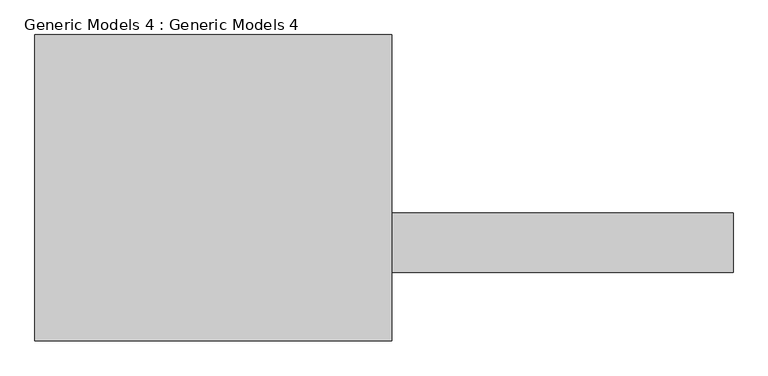
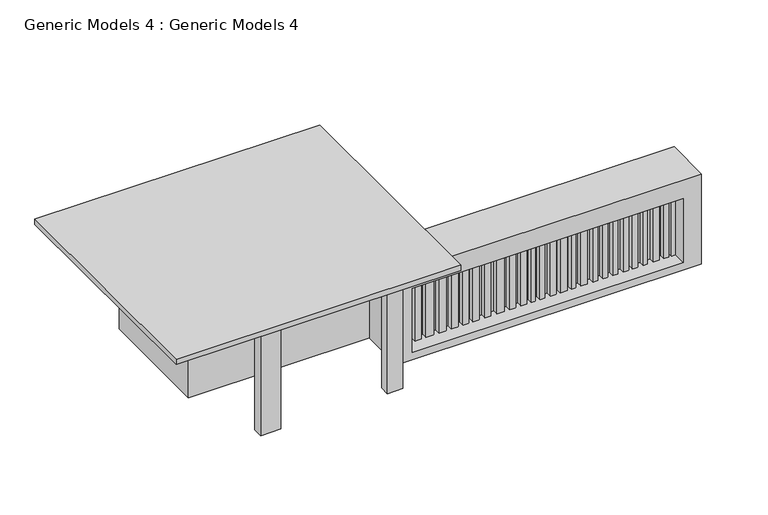
"""IFC4 building model written with IfcOpenShell, lengths in millimetres: proxy geometry, Generic Models 4 : Generic Models 4."""

from ifc_helpers import new_model, si_unit, frame, origin, place, context, project, spatial, polyline, outline, extrude, faceted_brep, source, transform, mapped, element, save


def generic_models_4_generic_models_4_f36dcc8b(model_context):
    return source(origin(), model_context, "Body", "SolidModel", [
        extrude(outline(polyline([(1788.9557244, -13852.2176249), (-4615.7230912, -13852.2176249), (-4615.7230912, -8353.4436591), (1788.9557244, -8353.4436591), (1788.9557244, -13852.2176249)])), frame((0.0, 0.0, 9144.0), z_axis=(0.0, 0.0, 1.0), x_axis=(1.0, 0.0, 0.0)), (0.0, 0.0, 1.0), 127.0),
        extrude(outline(polyline([(413.7770384, -13376.4602599), (413.7770384, -13147.8602599), (763.5531931, -13147.8602599), (763.5531931, -13376.4602599), (413.7770384, -13376.4602599)])), frame((0.0, 0.0, 6400.8), z_axis=(0.0, 0.0, 1.0), x_axis=(1.0, 0.0, 0.0)), (0.0, 0.0, 1.0), 2743.2),
        extrude(outline(polyline([(-2439.060811, -13147.8602599), (-1981.860811, -13147.8602599), (-1981.860811, -13376.4602599), (-2439.060811, -13376.4602599), (-2439.060811, -13147.8602599)])), frame((0.0, 0.0, 6400.8), z_axis=(0.0, 0.0, 1.0), x_axis=(1.0, 0.0, 0.0)), (0.0, 0.0, 1.0), 2743.2),
        extrude(outline(polyline([(-3010.560811, -11553.8436591), (-3010.560811, -8857.8706536), (1058.1030034, -8857.8706536), (1058.1030034, -11553.8436591), (-3010.560811, -11553.8436591)])), frame((0.0, 0.0, 6400.8), z_axis=(0.0, 0.0, 1.0), x_axis=(1.0, 0.0, 0.0)), (0.0, 0.0, 1.0), 2743.2),
        faceted_brep([(1058.1030034, -12620.6436591, 8549.4766171), (7916.1030034, -12620.6436591, 8549.4766171), (7916.1030034, -11553.8436591, 8549.4766171), (1058.1030034, -11553.8436591, 8549.4766171), (1058.1030034, -12620.6436591, 6400.8), (1058.1030034, -11553.8436591, 6400.8), (7916.1030034, -11553.8436591, 6400.8), (7916.1030034, -12620.6436591, 6400.8), (7505.039189, -12620.6436591, 8103.1737426), (7505.039189, -12620.6436591, 6579.1737426), (1409.039189, -12620.6436591, 6579.1737426), (1409.039189, -12620.6436591, 8103.1737426), (1409.039189, -12315.8436591, 8103.1737426), (1409.039189, -12315.8436591, 6579.1737426), (1527.4997407, -12315.8436591, 6579.1737426), (1527.4997407, -12315.8436591, 8103.1737426), (7505.039189, -12315.8436591, 6579.1737426), (7505.039189, -12315.8436591, 8103.1737426), (7412.689646, -12315.8436591, 8103.1737426), (7412.689646, -12315.8436591, 6579.1737426), (1788.9557244, -12315.8436591, 8103.1737426), (1637.639189, -12315.8436591, 8103.1737426), (1637.639189, -12315.8436591, 6579.1737426), (1788.9557244, -12315.8436591, 6579.1737426), (2067.842107, -12315.8436591, 8103.1737426), (1893.5381178, -12315.8436591, 8103.1737426), (1893.5381178, -12315.8436591, 6579.1737426), (2067.842107, -12315.8436591, 6579.1737426), (2346.7284896, -12315.8436591, 8103.1737426), (2181.1396999, -12315.8436591, 8103.1737426), (2181.1396999, -12315.8436591, 6579.1737426), (2346.7284896, -12315.8436591, 6579.1737426), (2616.8996727, -12315.8436591, 8103.1737426), (2460.0260825, -12315.8436591, 8103.1737426), (2460.0260825, -12315.8436591, 6579.1737426), (2616.8996727, -12315.8436591, 6579.1737426), (2860.9252575, -12315.8436591, 8103.1737426), (2721.4820662, -12315.8436591, 8103.1737426), (2721.4820662, -12315.8436591, 6579.1737426), (2860.9252575, -12315.8436591, 6579.1737426), (3087.5204434, -12315.8436591, 8103.1737426), (2948.0772521, -12315.8436591, 8103.1737426), (2948.0772521, -12315.8436591, 6579.1737426), (3087.5204434, -12315.8436591, 6579.1737426), (3348.976427, -12315.8436591, 8103.1737426), (3218.2484352, -12315.8436591, 8103.1737426), (3218.2484352, -12315.8436591, 6579.1737426), (3348.976427, -12315.8436591, 6579.1737426), (3656.939189, -12315.8436591, 8103.1737426), (3488.4196184, -12315.8436591, 8103.1737426), (3488.4196184, -12315.8436591, 6579.1737426), (3656.939189, -12315.8436591, 6579.1737426), (3915.4643917, -12315.8436591, 8103.1737426), (3767.306001, -12315.8436591, 8103.1737426), (3767.306001, -12315.8436591, 6579.1737426), (3915.4643917, -12315.8436591, 6579.1737426), (4159.4899765, -12315.8436591, 8103.1737426), (4028.7619846, -12315.8436591, 8103.1737426), (4028.7619846, -12315.8436591, 6579.1737426), (4159.4899765, -12315.8436591, 6579.1737426), (4357.287112, -12315.8436591, 8103.1737426), (4264.07237, -12315.8436591, 8103.1737426), (4264.07237, -12315.8436591, 6579.1737426), (4357.287112, -12315.8436591, 6579.1737426), (4569.4832727, -12315.8436591, 8103.1737426), (4457.039189, -12315.8436591, 8103.1737426), (4457.039189, -12315.8436591, 6579.1737426), (4569.4832727, -12315.8436591, 6579.1737426), (4819.5716049, -12315.8436591, 8103.1737426), (4690.7382216, -12315.8436591, 8103.1737426), (4690.7382216, -12315.8436591, 6579.1737426), (4819.5716049, -12315.8436591, 6579.1737426), (5077.2383714, -12315.8436591, 8103.1737426), (4910.5128166, -12315.8436591, 8103.1737426), (4910.5128166, -12315.8436591, 6579.1737426), (5077.2383714, -12315.8436591, 6579.1737426), (5266.6992292, -12315.8436591, 8103.1737426), (5160.6011488, -12315.8436591, 8103.1737426), (5160.6011488, -12315.8436591, 6579.1737426), (5266.6992292, -12315.8436591, 6579.1737426), (5524.3659957, -12315.8436591, 8103.1737426), (5380.3757438, -12315.8436591, 8103.1737426), (5380.3757438, -12315.8436591, 6579.1737426), (5524.3659957, -12315.8436591, 6579.1737426), (5759.2974593, -12315.8436591, 8103.1737426), (5645.6209447, -12315.8436591, 8103.1737426), (5645.6209447, -12315.8436591, 6579.1737426), (5759.2974593, -12315.8436591, 6579.1737426), (5979.0720543, -12315.8436591, 8103.1737426), (5872.973974, -12315.8436591, 8103.1737426), (5872.973974, -12315.8436591, 6579.1737426), (5979.0720543, -12315.8436591, 6579.1737426), (6206.4250836, -12315.8436591, 8103.1737426), (6095.339189, -12315.8436591, 8103.1737426), (6095.339189, -12315.8436591, 6579.1737426), (6206.4250836, -12315.8436591, 6579.1737426), (6456.5134158, -12315.8436591, 8103.1737426), (6327.6800326, -12315.8436591, 8103.1737426), (6327.6800326, -12315.8436591, 6579.1737426), (6456.5134158, -12315.8436591, 6579.1737426), (6661.1311422, -12315.8436591, 8103.1737426), (6539.8761932, -12315.8436591, 8103.1737426), (6539.8761932, -12315.8436591, 6579.1737426), (6661.1311422, -12315.8436591, 6579.1737426), (6873.3273029, -12315.8436591, 8103.1737426), (6782.3860912, -12315.8436591, 8103.1737426), (6782.3860912, -12315.8436591, 6579.1737426), (6873.3273029, -12315.8436591, 6579.1737426), (7146.150938, -12315.8436591, 8103.1737426), (7009.7391205, -12315.8436591, 8103.1737426), (7009.7391205, -12315.8436591, 6579.1737426), (7146.150938, -12315.8436591, 6579.1737426), (7350.7686644, -12315.8436591, 8103.1737426), (7244.6705841, -12315.8436591, 8103.1737426), (7244.6705841, -12315.8436591, 6579.1737426), (7350.7686644, -12315.8436591, 6579.1737426), (7412.689646, -12188.8436591, 6579.1737426), (7350.7686644, -12188.8436591, 6579.1737426), (7244.6705841, -12188.8436591, 6579.1737426), (7146.150938, -12188.8436591, 6579.1737426), (7009.7391205, -12188.8436591, 6579.1737426), (6873.3273029, -12188.8436591, 6579.1737426), (6782.3860912, -12188.8436591, 6579.1737426), (6661.1311422, -12188.8436591, 6579.1737426), (6539.8761932, -12188.8436591, 6579.1737426), (6456.5134158, -12188.8436591, 6579.1737426), (6327.6800326, -12188.8436591, 6579.1737426), (6206.4250836, -12188.8436591, 6579.1737426), (6095.339189, -12188.8436591, 6579.1737426), (5979.0720543, -12188.8436591, 6579.1737426), (5872.973974, -12188.8436591, 6579.1737426), (5759.2974593, -12188.8436591, 6579.1737426), (5645.6209447, -12188.8436591, 6579.1737426), (5524.3659957, -12188.8436591, 6579.1737426), (5380.3757438, -12188.8436591, 6579.1737426), (5266.6992292, -12188.8436591, 6579.1737426), (5160.6011488, -12188.8436591, 6579.1737426), (5077.2383714, -12188.8436591, 6579.1737426), (4910.5128166, -12188.8436591, 6579.1737426), (4819.5716049, -12188.8436591, 6579.1737426), (4690.7382216, -12188.8436591, 6579.1737426), (4569.4832727, -12188.8436591, 6579.1737426), (4457.039189, -12188.8436591, 6579.1737426), (4357.287112, -12188.8436591, 6579.1737426), (4264.07237, -12188.8436591, 6579.1737426), (4159.4899765, -12188.8436591, 6579.1737426), (4028.7619846, -12188.8436591, 6579.1737426), (3915.4643917, -12188.8436591, 6579.1737426), (3767.306001, -12188.8436591, 6579.1737426), (3656.939189, -12188.8436591, 6579.1737426), (3488.4196184, -12188.8436591, 6579.1737426), (3348.976427, -12188.8436591, 6579.1737426), (3218.2484352, -12188.8436591, 6579.1737426), (3087.5204434, -12188.8436591, 6579.1737426), (2948.0772521, -12188.8436591, 6579.1737426), (2860.9252575, -12188.8436591, 6579.1737426), (2721.4820662, -12188.8436591, 6579.1737426), (2616.8996727, -12188.8436591, 6579.1737426), (2460.0260825, -12188.8436591, 6579.1737426), (2346.7284896, -12188.8436591, 6579.1737426), (2181.1396999, -12188.8436591, 6579.1737426), (2067.842107, -12188.8436591, 6579.1737426), (1893.5381178, -12188.8436591, 6579.1737426), (1788.9557244, -12188.8436591, 6579.1737426), (1637.639189, -12188.8436591, 6579.1737426), (1527.4997407, -12188.8436591, 6579.1737426), (1527.4997407, -12188.8436591, 8103.1737426), (1637.639189, -12188.8436591, 8103.1737426), (1788.9557244, -12188.8436591, 8103.1737426), (1893.5381178, -12188.8436591, 8103.1737426), (2067.842107, -12188.8436591, 8103.1737426), (2181.1396999, -12188.8436591, 8103.1737426), (2346.7284896, -12188.8436591, 8103.1737426), (2460.0260825, -12188.8436591, 8103.1737426), (2616.8996727, -12188.8436591, 8103.1737426), (2721.4820662, -12188.8436591, 8103.1737426), (2860.9252575, -12188.8436591, 8103.1737426), (2948.0772521, -12188.8436591, 8103.1737426), (3087.5204434, -12188.8436591, 8103.1737426), (3218.2484352, -12188.8436591, 8103.1737426), (3348.976427, -12188.8436591, 8103.1737426), (3488.4196184, -12188.8436591, 8103.1737426), (3656.939189, -12188.8436591, 8103.1737426), (3767.306001, -12188.8436591, 8103.1737426), (3915.4643917, -12188.8436591, 8103.1737426), (4028.7619846, -12188.8436591, 8103.1737426), (4159.4899765, -12188.8436591, 8103.1737426), (4264.07237, -12188.8436591, 8103.1737426), (4357.287112, -12188.8436591, 8103.1737426), (4457.039189, -12188.8436591, 8103.1737426), (4569.4832727, -12188.8436591, 8103.1737426), (4690.7382216, -12188.8436591, 8103.1737426), (4819.5716049, -12188.8436591, 8103.1737426), (4910.5128166, -12188.8436591, 8103.1737426), (5077.2383714, -12188.8436591, 8103.1737426), (5160.6011488, -12188.8436591, 8103.1737426), (5266.6992292, -12188.8436591, 8103.1737426), (5380.3757438, -12188.8436591, 8103.1737426), (5524.3659957, -12188.8436591, 8103.1737426), (5645.6209447, -12188.8436591, 8103.1737426), (5759.2974593, -12188.8436591, 8103.1737426), (5872.973974, -12188.8436591, 8103.1737426), (5979.0720543, -12188.8436591, 8103.1737426), (6095.339189, -12188.8436591, 8103.1737426), (6206.4250836, -12188.8436591, 8103.1737426), (6327.6800326, -12188.8436591, 8103.1737426), (6456.5134158, -12188.8436591, 8103.1737426), (6539.8761932, -12188.8436591, 8103.1737426), (6661.1311422, -12188.8436591, 8103.1737426), (6782.3860912, -12188.8436591, 8103.1737426), (6873.3273029, -12188.8436591, 8103.1737426), (7009.7391205, -12188.8436591, 8103.1737426), (7146.150938, -12188.8436591, 8103.1737426), (7244.6705841, -12188.8436591, 8103.1737426), (7350.7686644, -12188.8436591, 8103.1737426), (7412.689646, -12188.8436591, 8103.1737426)], [[[0, 1, 2, 3]], [[4, 5, 6, 7]], [[1, 0, 4, 7], [8, 9, 10, 11]], [[2, 1, 7, 6]], [[3, 2, 6, 5]], [[0, 3, 5, 4]], [[12, 13, 14, 15]], [[16, 17, 18, 19]], [[20, 21, 22, 23]], [[24, 25, 26, 27]], [[28, 29, 30, 31]], [[32, 33, 34, 35]], [[36, 37, 38, 39]], [[40, 41, 42, 43]], [[44, 45, 46, 47]], [[48, 49, 50, 51]], [[52, 53, 54, 55]], [[56, 57, 58, 59]], [[60, 61, 62, 63]], [[64, 65, 66, 67]], [[68, 69, 70, 71]], [[72, 73, 74, 75]], [[76, 77, 78, 79]], [[80, 81, 82, 83]], [[84, 85, 86, 87]], [[88, 89, 90, 91]], [[92, 93, 94, 95]], [[96, 97, 98, 99]], [[100, 101, 102, 103]], [[104, 105, 106, 107]], [[108, 109, 110, 111]], [[112, 113, 114, 115]], [[17, 16, 9, 8]], [[9, 16, 19, 116, 117, 115, 114, 118, 119, 111, 110, 120, 121, 107, 106, 122, 123, 103, 102, 124, 125, 99, 98, 126, 127, 95, 94, 128, 129, 91, 90, 130, 131, 87, 86, 132, 133, 83, 82, 134, 135, 79, 78, 136, 137, 75, 74, 138, 139, 71, 70, 140, 141, 67, 66, 142, 143, 63, 62, 144, 145, 59, 58, 146, 147, 55, 54, 148, 149, 51, 50, 150, 151, 47, 46, 152, 153, 43, 42, 154, 155, 39, 38, 156, 157, 35, 34, 158, 159, 31, 30, 160, 161, 27, 26, 162, 163, 23, 22, 164, 165, 14, 13, 10]], [[13, 12, 11, 10]], [[17, 8, 11, 12, 15, 166, 167, 21, 20, 168, 169, 25, 24, 170, 171, 29, 28, 172, 173, 33, 32, 174, 175, 37, 36, 176, 177, 41, 40, 178, 179, 45, 44, 180, 181, 49, 48, 182, 183, 53, 52, 184, 185, 57, 56, 186, 187, 61, 60, 188, 189, 65, 64, 190, 191, 69, 68, 192, 193, 73, 72, 194, 195, 77, 76, 196, 197, 81, 80, 198, 199, 85, 84, 200, 201, 89, 88, 202, 203, 93, 92, 204, 205, 97, 96, 206, 207, 101, 100, 208, 209, 105, 104, 210, 211, 109, 108, 212, 213, 113, 112, 214, 215, 18]], [[167, 166, 165, 164]], [[169, 168, 163, 162]], [[171, 170, 161, 160]], [[173, 172, 159, 158]], [[175, 174, 157, 156]], [[177, 176, 155, 154]], [[179, 178, 153, 152]], [[181, 180, 151, 150]], [[183, 182, 149, 148]], [[185, 184, 147, 146]], [[187, 186, 145, 144]], [[189, 188, 143, 142]], [[191, 190, 141, 140]], [[193, 192, 139, 138]], [[195, 194, 137, 136]], [[197, 196, 135, 134]], [[199, 198, 133, 132]], [[201, 200, 131, 130]], [[203, 202, 129, 128]], [[205, 204, 127, 126]], [[207, 206, 125, 124]], [[209, 208, 123, 122]], [[211, 210, 121, 120]], [[213, 212, 119, 118]], [[215, 214, 117, 116]], [[167, 164, 22, 21]], [[165, 166, 15, 14]], [[169, 162, 26, 25]], [[163, 168, 20, 23]], [[171, 160, 30, 29]], [[161, 170, 24, 27]], [[173, 158, 34, 33]], [[159, 172, 28, 31]], [[175, 156, 38, 37]], [[157, 174, 32, 35]], [[177, 154, 42, 41]], [[155, 176, 36, 39]], [[179, 152, 46, 45]], [[153, 178, 40, 43]], [[181, 150, 50, 49]], [[151, 180, 44, 47]], [[183, 148, 54, 53]], [[149, 182, 48, 51]], [[185, 146, 58, 57]], [[147, 184, 52, 55]], [[187, 144, 62, 61]], [[145, 186, 56, 59]], [[189, 142, 66, 65]], [[143, 188, 60, 63]], [[191, 140, 70, 69]], [[141, 190, 64, 67]], [[193, 138, 74, 73]], [[139, 192, 68, 71]], [[195, 136, 78, 77]], [[137, 194, 72, 75]], [[197, 134, 82, 81]], [[135, 196, 76, 79]], [[199, 132, 86, 85]], [[133, 198, 80, 83]], [[201, 130, 90, 89]], [[131, 200, 84, 87]], [[203, 128, 94, 93]], [[129, 202, 88, 91]], [[205, 126, 98, 97]], [[127, 204, 92, 95]], [[207, 124, 102, 101]], [[125, 206, 96, 99]], [[209, 122, 106, 105]], [[123, 208, 100, 103]], [[211, 120, 110, 109]], [[121, 210, 104, 107]], [[213, 118, 114, 113]], [[119, 212, 108, 111]], [[215, 116, 19, 18]], [[117, 214, 112, 115]]]),
    ])


if __name__ == "__main__":
    model = new_model("IFC4")
    model_context = context("Model", 3, world=origin())
    ifc_project = project(units=[si_unit("LENGTHUNIT", "METRE", prefix="MILLI")], contexts=[model_context])
    site = spatial("IfcSite", under=ifc_project)
    building = spatial("IfcBuilding", under=site)
    placement = place(None, origin())
    generic_models_4_generic_models_4_shape = generic_models_4_generic_models_4_f36dcc8b(model_context)
    element("IfcBuildingElementProxy", 1, Name="Generic Models 4 : Generic Models 4", ObjectType="Generic Models 4 : Generic Models 4", at=placement, inside=building, context=model_context, shape_type="MappedRepresentation", body=[
        mapped(generic_models_4_generic_models_4_shape, transform((0.0, 0.0, 0.0), x_axis=(1.0, 0.0, 0.0), y_axis=(0.0, 1.0, 0.0), z_axis=(0.0, 0.0, 1.0))),
    ])
    save(model, "model.ifc")
